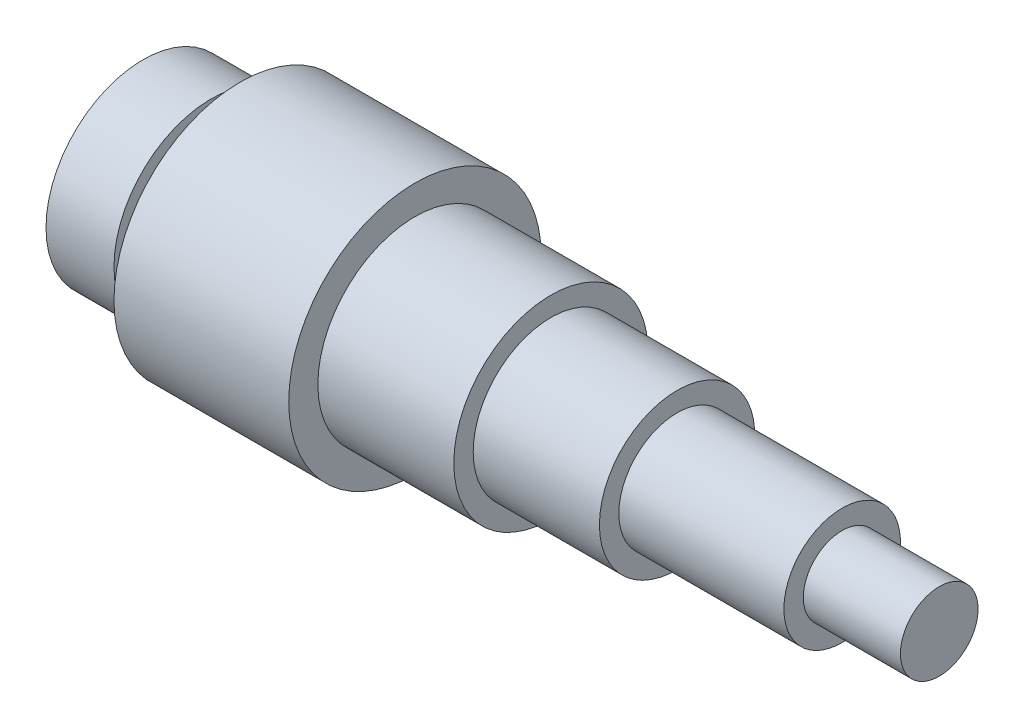
ISO-10303-21;
HEADER;
FILE_DESCRIPTION(('STEP AP214'),'2;1');
FILE_NAME('part.step','',(''),(''),'','','');
FILE_SCHEMA(('AUTOMOTIVE_DESIGN { 1 0 10303 214 1 1 1 1 }'));
ENDSEC;
DATA;
#1=APPLICATION_CONTEXT('core data for automotive mechanical design processes');
#2=APPLICATION_PROTOCOL_DEFINITION('international standard','automotive_design',2000,#1);
#3=PRODUCT_CONTEXT('',#1,'mechanical');
#4=PRODUCT('Part','Part','',(#3));
#5=PRODUCT_RELATED_PRODUCT_CATEGORY('part','',(#4));
#6=PRODUCT_DEFINITION_FORMATION('','',#4);
#7=PRODUCT_DEFINITION_CONTEXT('part definition',#1,'design');
#8=PRODUCT_DEFINITION('design','',#6,#7);
#9=PRODUCT_DEFINITION_SHAPE('','',#8);
#10=(LENGTH_UNIT() NAMED_UNIT(*) SI_UNIT(.MILLI.,.METRE.));
#11=(NAMED_UNIT(*) PLANE_ANGLE_UNIT() SI_UNIT($,.RADIAN.));
#12=(NAMED_UNIT(*) SI_UNIT($,.STERADIAN.) SOLID_ANGLE_UNIT());
#13=UNCERTAINTY_MEASURE_WITH_UNIT(LENGTH_MEASURE(1.E-05),#10,'distance_accuracy_value','');
#14=(GEOMETRIC_REPRESENTATION_CONTEXT(3) GLOBAL_UNCERTAINTY_ASSIGNED_CONTEXT((#13)) GLOBAL_UNIT_ASSIGNED_CONTEXT((#10,
#11,#12)) REPRESENTATION_CONTEXT('',''));
#15=CARTESIAN_POINT('',(0.,0.,0.));
#16=DIRECTION('',(0.,0.,1.));
#17=DIRECTION('',(1.,0.,0.));
#18=AXIS2_PLACEMENT_3D('',#15,#16,#17);
#19=CARTESIAN_POINT('',(0.,0.,0.));
#20=DIRECTION('',(1.,0.,0.));
#21=DIRECTION('',(0.,0.,-1.));
#22=AXIS2_PLACEMENT_3D('',#19,#20,#21);
#23=PLANE('',#22);
#24=CARTESIAN_POINT('',(0.,0.,0.));
#25=DIRECTION('',(-1.,0.,0.));
#26=DIRECTION('',(0.,0.,1.));
#27=AXIS2_PLACEMENT_3D('',#24,#25,#26);
#28=CIRCLE('',#27,2.775);
#29=CARTESIAN_POINT('',(0.,0.,2.775));
#30=VERTEX_POINT('',#29);
#31=EDGE_CURVE('E70',#30,#30,#28,.T.);
#32=ORIENTED_EDGE('',*,*,#31,.F.);
#33=EDGE_LOOP('',(#32));
#34=FACE_BOUND('',#33,.T.);
#35=CARTESIAN_POINT('',(0.,0.,0.));
#36=DIRECTION('',(-1.,0.,0.));
#37=DIRECTION('',(0.,0.,1.));
#38=AXIS2_PLACEMENT_3D('',#35,#36,#37);
#39=CIRCLE('',#38,10.);
#40=CARTESIAN_POINT('',(0.,0.,10.));
#41=VERTEX_POINT('',#40);
#42=EDGE_CURVE('E11',#41,#41,#39,.T.);
#43=ORIENTED_EDGE('',*,*,#42,.T.);
#44=EDGE_LOOP('',(#43));
#45=FACE_BOUND('',#44,.T.);
#46=ADVANCED_FACE('F41',(#34,#45),#23,.F.);
#47=CARTESIAN_POINT('',(-602.79260317363,0.,0.));
#48=DIRECTION('',(-1.,0.,0.));
#49=DIRECTION('',(0.,0.,1.));
#50=AXIS2_PLACEMENT_3D('',#47,#48,#49);
#51=CYLINDRICAL_SURFACE('',#50,10.);
#52=ORIENTED_EDGE('',*,*,#42,.F.);
#53=EDGE_LOOP('',(#52));
#54=FACE_BOUND('',#53,.T.);
#55=CARTESIAN_POINT('',(7.00000000000001,0.,0.));
#56=DIRECTION('',(-1.,0.,0.));
#57=DIRECTION('',(0.,0.,1.));
#58=AXIS2_PLACEMENT_3D('',#55,#56,#57);
#59=CIRCLE('',#58,10.);
#60=CARTESIAN_POINT('',(7.00000000000001,0.,10.));
#61=VERTEX_POINT('',#60);
#62=EDGE_CURVE('E50',#61,#61,#59,.T.);
#63=ORIENTED_EDGE('',*,*,#62,.T.);
#64=EDGE_LOOP('',(#63));
#65=FACE_BOUND('',#64,.T.);
#66=ADVANCED_FACE('F104',(#54,#65),#51,.T.);
#67=CARTESIAN_POINT('',(7.,10.,0.));
#68=DIRECTION('',(-1.,0.,0.));
#69=DIRECTION('',(0.,0.,1.));
#70=AXIS2_PLACEMENT_3D('',#67,#68,#69);
#71=PLANE('',#70);
#72=ORIENTED_EDGE('',*,*,#62,.F.);
#73=EDGE_LOOP('',(#72));
#74=FACE_BOUND('',#73,.T.);
#75=CARTESIAN_POINT('',(7.00000000000001,0.,0.));
#76=DIRECTION('',(-1.,0.,0.));
#77=DIRECTION('',(0.,0.,1.));
#78=AXIS2_PLACEMENT_3D('',#75,#76,#77);
#79=CIRCLE('',#78,8.);
#80=CARTESIAN_POINT('',(7.00000000000001,0.,8.));
#81=VERTEX_POINT('',#80);
#82=EDGE_CURVE('E99',#81,#81,#79,.T.);
#83=ORIENTED_EDGE('',*,*,#82,.T.);
#84=EDGE_LOOP('',(#83));
#85=FACE_BOUND('',#84,.T.);
#86=ADVANCED_FACE('F110',(#74,#85),#71,.F.);
#87=CARTESIAN_POINT('',(-602.79260317363,0.,0.));
#88=DIRECTION('',(-1.,0.,0.));
#89=DIRECTION('',(0.,0.,1.));
#90=AXIS2_PLACEMENT_3D('',#87,#88,#89);
#91=CYLINDRICAL_SURFACE('',#90,8.);
#92=ORIENTED_EDGE('',*,*,#82,.F.);
#93=EDGE_LOOP('',(#92));
#94=FACE_BOUND('',#93,.T.);
#95=CARTESIAN_POINT('',(10.,0.,0.));
#96=DIRECTION('',(-1.,0.,0.));
#97=DIRECTION('',(0.,0.,1.));
#98=AXIS2_PLACEMENT_3D('',#95,#96,#97);
#99=CIRCLE('',#98,8.);
#100=CARTESIAN_POINT('',(10.,0.,8.));
#101=VERTEX_POINT('',#100);
#102=EDGE_CURVE('E100',#101,#101,#99,.T.);
#103=ORIENTED_EDGE('',*,*,#102,.T.);
#104=EDGE_LOOP('',(#103));
#105=FACE_BOUND('',#104,.T.);
#106=ADVANCED_FACE('F109',(#94,#105),#91,.T.);
#107=CARTESIAN_POINT('',(10.,8.,0.));
#108=DIRECTION('',(1.,0.,0.));
#109=DIRECTION('',(0.,0.,-1.));
#110=AXIS2_PLACEMENT_3D('',#107,#108,#109);
#111=PLANE('',#110);
#112=ORIENTED_EDGE('',*,*,#102,.F.);
#113=EDGE_LOOP('',(#112));
#114=FACE_BOUND('',#113,.T.);
#115=CARTESIAN_POINT('',(10.,0.,0.));
#116=DIRECTION('',(-1.,0.,0.));
#117=DIRECTION('',(0.,0.,1.));
#118=AXIS2_PLACEMENT_3D('',#115,#116,#117);
#119=CIRCLE('',#118,13.);
#120=CARTESIAN_POINT('',(10.,0.,13.));
#121=VERTEX_POINT('',#120);
#122=EDGE_CURVE('E94',#121,#121,#119,.T.);
#123=ORIENTED_EDGE('',*,*,#122,.T.);
#124=EDGE_LOOP('',(#123));
#125=FACE_BOUND('',#124,.T.);
#126=ADVANCED_FACE('F119',(#114,#125),#111,.F.);
#127=CARTESIAN_POINT('',(-602.79260317363,0.,0.));
#128=DIRECTION('',(-1.,0.,0.));
#129=DIRECTION('',(0.,0.,1.));
#130=AXIS2_PLACEMENT_3D('',#127,#128,#129);
#131=CYLINDRICAL_SURFACE('',#130,13.);
#132=ORIENTED_EDGE('',*,*,#122,.F.);
#133=EDGE_LOOP('',(#132));
#134=FACE_BOUND('',#133,.T.);
#135=CARTESIAN_POINT('',(28.,0.,0.));
#136=DIRECTION('',(-1.,0.,0.));
#137=DIRECTION('',(0.,0.,1.));
#138=AXIS2_PLACEMENT_3D('',#135,#136,#137);
#139=CIRCLE('',#138,13.);
#140=CARTESIAN_POINT('',(28.,0.,13.));
#141=VERTEX_POINT('',#140);
#142=EDGE_CURVE('E93',#141,#141,#139,.T.);
#143=ORIENTED_EDGE('',*,*,#142,.T.);
#144=EDGE_LOOP('',(#143));
#145=FACE_BOUND('',#144,.T.);
#146=ADVANCED_FACE('F125',(#134,#145),#131,.T.);
#147=CARTESIAN_POINT('',(28.,13.,0.));
#148=DIRECTION('',(-1.,0.,0.));
#149=DIRECTION('',(0.,0.,1.));
#150=AXIS2_PLACEMENT_3D('',#147,#148,#149);
#151=PLANE('',#150);
#152=ORIENTED_EDGE('',*,*,#142,.F.);
#153=EDGE_LOOP('',(#152));
#154=FACE_BOUND('',#153,.T.);
#155=CARTESIAN_POINT('',(28.,0.,0.));
#156=DIRECTION('',(-1.,0.,0.));
#157=DIRECTION('',(0.,0.,1.));
#158=AXIS2_PLACEMENT_3D('',#155,#156,#157);
#159=CIRCLE('',#158,10.);
#160=CARTESIAN_POINT('',(28.,0.,10.));
#161=VERTEX_POINT('',#160);
#162=EDGE_CURVE('E86',#161,#161,#159,.T.);
#163=ORIENTED_EDGE('',*,*,#162,.T.);
#164=EDGE_LOOP('',(#163));
#165=FACE_BOUND('',#164,.T.);
#166=ADVANCED_FACE('F126',(#154,#165),#151,.F.);
#167=CARTESIAN_POINT('',(-602.79260317363,0.,0.));
#168=DIRECTION('',(-1.,0.,0.));
#169=DIRECTION('',(0.,0.,1.));
#170=AXIS2_PLACEMENT_3D('',#167,#168,#169);
#171=CYLINDRICAL_SURFACE('',#170,10.);
#172=ORIENTED_EDGE('',*,*,#162,.F.);
#173=EDGE_LOOP('',(#172));
#174=FACE_BOUND('',#173,.T.);
#175=CARTESIAN_POINT('',(42.,0.,0.));
#176=DIRECTION('',(-1.,0.,0.));
#177=DIRECTION('',(0.,0.,1.));
#178=AXIS2_PLACEMENT_3D('',#175,#176,#177);
#179=CIRCLE('',#178,10.);
#180=CARTESIAN_POINT('',(42.,0.,10.));
#181=VERTEX_POINT('',#180);
#182=EDGE_CURVE('E83',#181,#181,#179,.T.);
#183=ORIENTED_EDGE('',*,*,#182,.T.);
#184=EDGE_LOOP('',(#183));
#185=FACE_BOUND('',#184,.T.);
#186=ADVANCED_FACE('F133',(#174,#185),#171,.T.);
#187=CARTESIAN_POINT('',(42.,10.,0.));
#188=DIRECTION('',(-1.,0.,0.));
#189=DIRECTION('',(0.,0.,1.));
#190=AXIS2_PLACEMENT_3D('',#187,#188,#189);
#191=PLANE('',#190);
#192=ORIENTED_EDGE('',*,*,#182,.F.);
#193=EDGE_LOOP('',(#192));
#194=FACE_BOUND('',#193,.T.);
#195=CARTESIAN_POINT('',(42.,0.,0.));
#196=DIRECTION('',(-1.,0.,0.));
#197=DIRECTION('',(0.,0.,1.));
#198=AXIS2_PLACEMENT_3D('',#195,#196,#197);
#199=CIRCLE('',#198,8.);
#200=CARTESIAN_POINT('',(42.,0.,8.));
#201=VERTEX_POINT('',#200);
#202=EDGE_CURVE('E85',#201,#201,#199,.T.);
#203=ORIENTED_EDGE('',*,*,#202,.T.);
#204=EDGE_LOOP('',(#203));
#205=FACE_BOUND('',#204,.T.);
#206=ADVANCED_FACE('F138',(#194,#205),#191,.F.);
#207=CARTESIAN_POINT('',(-602.79260317363,0.,0.));
#208=DIRECTION('',(-1.,0.,0.));
#209=DIRECTION('',(0.,0.,1.));
#210=AXIS2_PLACEMENT_3D('',#207,#208,#209);
#211=CYLINDRICAL_SURFACE('',#210,8.);
#212=ORIENTED_EDGE('',*,*,#202,.F.);
#213=EDGE_LOOP('',(#212));
#214=FACE_BOUND('',#213,.T.);
#215=CARTESIAN_POINT('',(55.,0.,0.));
#216=DIRECTION('',(-1.,0.,0.));
#217=DIRECTION('',(0.,0.,1.));
#218=AXIS2_PLACEMENT_3D('',#215,#216,#217);
#219=CIRCLE('',#218,8.);
#220=CARTESIAN_POINT('',(55.,0.,8.));
#221=VERTEX_POINT('',#220);
#222=EDGE_CURVE('E78',#221,#221,#219,.T.);
#223=ORIENTED_EDGE('',*,*,#222,.T.);
#224=EDGE_LOOP('',(#223));
#225=FACE_BOUND('',#224,.T.);
#226=ADVANCED_FACE('F148',(#214,#225),#211,.T.);
#227=CARTESIAN_POINT('',(55.,8.,0.));
#228=DIRECTION('',(-1.,0.,0.));
#229=DIRECTION('',(0.,0.,1.));
#230=AXIS2_PLACEMENT_3D('',#227,#228,#229);
#231=PLANE('',#230);
#232=ORIENTED_EDGE('',*,*,#222,.F.);
#233=EDGE_LOOP('',(#232));
#234=FACE_BOUND('',#233,.T.);
#235=CARTESIAN_POINT('',(55.,0.,0.));
#236=DIRECTION('',(-1.,0.,0.));
#237=DIRECTION('',(0.,0.,1.));
#238=AXIS2_PLACEMENT_3D('',#235,#236,#237);
#239=CIRCLE('',#238,6.);
#240=CARTESIAN_POINT('',(55.,0.,6.));
#241=VERTEX_POINT('',#240);
#242=EDGE_CURVE('E79',#241,#241,#239,.T.);
#243=ORIENTED_EDGE('',*,*,#242,.T.);
#244=EDGE_LOOP('',(#243));
#245=FACE_BOUND('',#244,.T.);
#246=ADVANCED_FACE('F155',(#234,#245),#231,.F.);
#247=CARTESIAN_POINT('',(-602.79260317363,0.,0.));
#248=DIRECTION('',(-1.,0.,0.));
#249=DIRECTION('',(0.,0.,1.));
#250=AXIS2_PLACEMENT_3D('',#247,#248,#249);
#251=CYLINDRICAL_SURFACE('',#250,6.);
#252=ORIENTED_EDGE('',*,*,#242,.F.);
#253=EDGE_LOOP('',(#252));
#254=FACE_BOUND('',#253,.T.);
#255=CARTESIAN_POINT('',(72.,0.,0.));
#256=DIRECTION('',(-1.,0.,0.));
#257=DIRECTION('',(0.,0.,1.));
#258=AXIS2_PLACEMENT_3D('',#255,#256,#257);
#259=CIRCLE('',#258,6.);
#260=CARTESIAN_POINT('',(72.,0.,6.));
#261=VERTEX_POINT('',#260);
#262=EDGE_CURVE('E71',#261,#261,#259,.T.);
#263=ORIENTED_EDGE('',*,*,#262,.T.);
#264=EDGE_LOOP('',(#263));
#265=FACE_BOUND('',#264,.T.);
#266=ADVANCED_FACE('F158',(#254,#265),#251,.T.);
#267=CARTESIAN_POINT('',(72.,6.,0.));
#268=DIRECTION('',(-1.,0.,0.));
#269=DIRECTION('',(0.,0.,1.));
#270=AXIS2_PLACEMENT_3D('',#267,#268,#269);
#271=PLANE('',#270);
#272=ORIENTED_EDGE('',*,*,#262,.F.);
#273=EDGE_LOOP('',(#272));
#274=FACE_BOUND('',#273,.T.);
#275=CARTESIAN_POINT('',(72.,0.,0.));
#276=DIRECTION('',(-1.,0.,0.));
#277=DIRECTION('',(0.,0.,1.));
#278=AXIS2_PLACEMENT_3D('',#275,#276,#277);
#279=CIRCLE('',#278,4.);
#280=CARTESIAN_POINT('',(72.,0.,4.));
#281=VERTEX_POINT('',#280);
#282=EDGE_CURVE('E63',#281,#281,#279,.T.);
#283=ORIENTED_EDGE('',*,*,#282,.T.);
#284=EDGE_LOOP('',(#283));
#285=FACE_BOUND('',#284,.T.);
#286=ADVANCED_FACE('F163',(#274,#285),#271,.F.);
#287=CARTESIAN_POINT('',(-602.79260317363,0.,0.));
#288=DIRECTION('',(-1.,0.,0.));
#289=DIRECTION('',(0.,0.,1.));
#290=AXIS2_PLACEMENT_3D('',#287,#288,#289);
#291=CYLINDRICAL_SURFACE('',#290,4.);
#292=ORIENTED_EDGE('',*,*,#282,.F.);
#293=EDGE_LOOP('',(#292));
#294=FACE_BOUND('',#293,.T.);
#295=CARTESIAN_POINT('',(82.,0.,0.));
#296=DIRECTION('',(-1.,0.,0.));
#297=DIRECTION('',(0.,0.,1.));
#298=AXIS2_PLACEMENT_3D('',#295,#296,#297);
#299=CIRCLE('',#298,4.);
#300=CARTESIAN_POINT('',(82.,0.,4.));
#301=VERTEX_POINT('',#300);
#302=EDGE_CURVE('E58',#301,#301,#299,.T.);
#303=ORIENTED_EDGE('',*,*,#302,.T.);
#304=EDGE_LOOP('',(#303));
#305=FACE_BOUND('',#304,.T.);
#306=ADVANCED_FACE('F168',(#294,#305),#291,.T.);
#307=CARTESIAN_POINT('',(82.0000000000034,4.,0.));
#308=DIRECTION('',(-1.,0.,0.));
#309=DIRECTION('',(0.,0.,1.));
#310=AXIS2_PLACEMENT_3D('',#307,#308,#309);
#311=PLANE('',#310);
#312=ORIENTED_EDGE('',*,*,#302,.F.);
#313=EDGE_LOOP('',(#312));
#314=FACE_BOUND('',#313,.T.);
#315=ADVANCED_FACE('F53',(#314),#311,.F.);
#316=CARTESIAN_POINT('',(36.3476332976742,0.,0.));
#317=DIRECTION('',(-1.,0.,0.));
#318=DIRECTION('',(0.,0.,1.));
#319=AXIS2_PLACEMENT_3D('',#316,#317,#318);
#320=CONICAL_SURFACE('',#319,2.74999999999999,1.02974425867665);
#321=CARTESIAN_POINT('',(38.,0.,0.));
#322=VERTEX_POINT('',#321);
#323=VERTEX_LOOP('',#322);
#324=FACE_BOUND('',#323,.T.);
#325=CARTESIAN_POINT('',(36.3476332976742,0.,0.));
#326=DIRECTION('',(-1.,0.,0.));
#327=DIRECTION('',(0.,0.,1.));
#328=AXIS2_PLACEMENT_3D('',#325,#326,#327);
#329=CIRCLE('',#328,2.74999999999999);
#330=CARTESIAN_POINT('',(36.3476332976742,0.,2.74999999999999));
#331=VERTEX_POINT('',#330);
#332=EDGE_CURVE('E59',#331,#331,#329,.T.);
#333=ORIENTED_EDGE('',*,*,#332,.T.);
#334=EDGE_LOOP('',(#333));
#335=FACE_BOUND('',#334,.T.);
#336=ADVANCED_FACE('F49',(#324,#335),#320,.F.);
#337=CARTESIAN_POINT('',(0.,0.,0.));
#338=DIRECTION('',(-1.,0.,0.));
#339=DIRECTION('',(0.,0.,1.));
#340=AXIS2_PLACEMENT_3D('',#337,#338,#339);
#341=CYLINDRICAL_SURFACE('',#340,2.74999999999999);
#342=ORIENTED_EDGE('',*,*,#332,.F.);
#343=EDGE_LOOP('',(#342));
#344=FACE_BOUND('',#343,.T.);
#345=CARTESIAN_POINT('',(0.0209774907794363,0.,0.));
#346=DIRECTION('',(-1.,0.,0.));
#347=DIRECTION('',(0.,0.,1.));
#348=AXIS2_PLACEMENT_3D('',#345,#346,#347);
#349=CIRCLE('',#348,2.75);
#350=CARTESIAN_POINT('',(0.0209774907794363,0.,2.75));
#351=VERTEX_POINT('',#350);
#352=EDGE_CURVE('E64',#351,#351,#349,.T.);
#353=ORIENTED_EDGE('',*,*,#352,.T.);
#354=EDGE_LOOP('',(#353));
#355=FACE_BOUND('',#354,.T.);
#356=ADVANCED_FACE('F52',(#344,#355),#341,.F.);
#357=CARTESIAN_POINT('',(0.,0.,0.));
#358=DIRECTION('',(-1.,0.,0.));
#359=DIRECTION('',(0.,0.,1.));
#360=AXIS2_PLACEMENT_3D('',#357,#358,#359);
#361=CONICAL_SURFACE('',#360,2.775,0.872664625997154);
#362=ORIENTED_EDGE('',*,*,#352,.F.);
#363=EDGE_LOOP('',(#362));
#364=FACE_BOUND('',#363,.T.);
#365=ORIENTED_EDGE('',*,*,#31,.T.);
#366=EDGE_LOOP('',(#365));
#367=FACE_BOUND('',#366,.T.);
#368=ADVANCED_FACE('F191',(#364,#367),#361,.F.);
#369=CLOSED_SHELL('',(#46,#66,#86,#106,#126,#146,#166,#186,#206,#226,#246,#266,#286,#306,#315,
#336,#356,#368));
#370=MANIFOLD_SOLID_BREP('B2',#369);
#371=ADVANCED_BREP_SHAPE_REPRESENTATION('',(#18,#370),#14);
#372=SHAPE_DEFINITION_REPRESENTATION(#9,#371);
ENDSEC;
END-ISO-10303-21;
